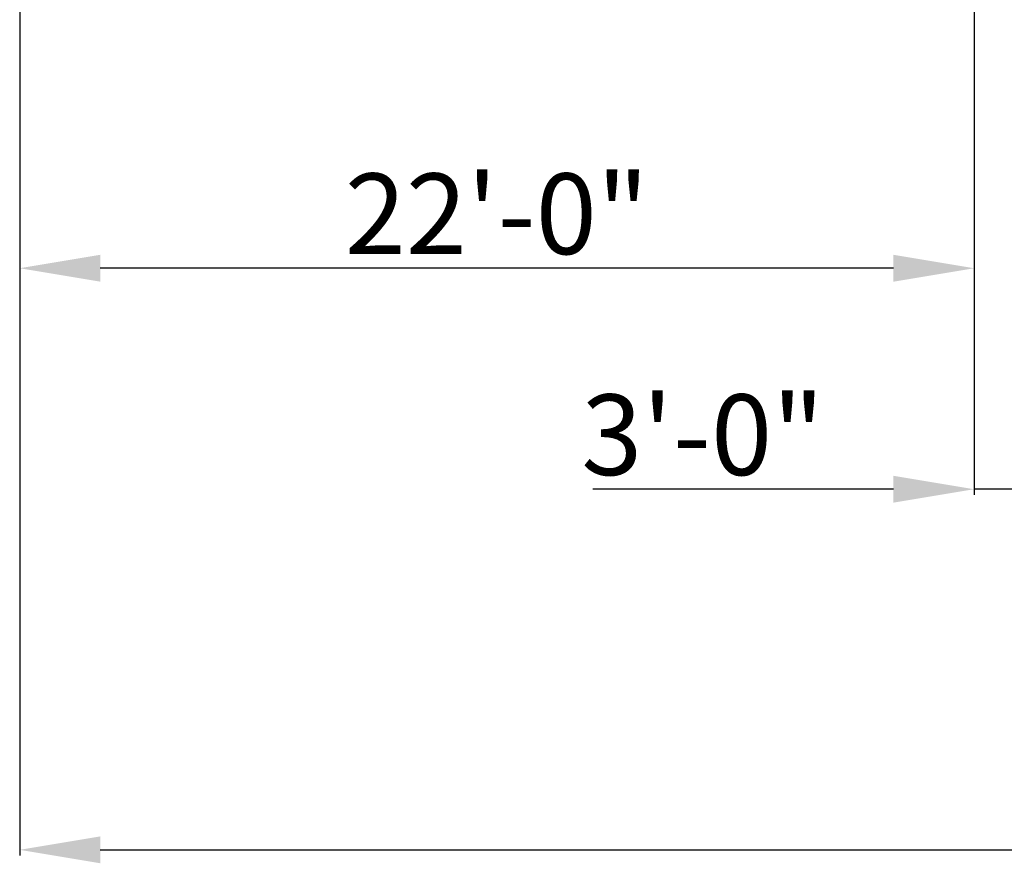
# Model space of a CAD drawing. Units: inches. Extents: x 2043 to 3177, y 1429 to 2563.
# Tile 1 of 14: x 2234 to 2453, y 1429 to 1617. Entities that reach past the tile are written whole.
import ezdxf

# ---------------------------------------------------------------- set-up
doc = ezdxf.new("R2010")
doc.units = ezdxf.units.IN
doc.layers.add('A-ANNO-DIMS', color=2, linetype='Continuous', lineweight=13)
doc.styles.get("Standard").update_dxf_attribs({"font": 'arial.ttf'})
doc.dimstyles.new('ISO-25', dxfattribs={"dimtxt": 18, "dimasz": 18, "dimexe": 1.25, "dimexo": 0.625, "dimtad": 1, "dimlunit": 3, "dimtxsty": 'Standard', "dimcen": 2.5, "dimadec": 0, "dimazin": 0, "dimtfac": 1, "dimtmove": 0, "dimatfit": 3, "dimfxl": 1, "dimarcsym": 0})

# ---------------------------------------------------------------- blocks, each defined once
blk = doc.blocks.new('*D23')
at = {"layer": 'A-ANNO-DIMS', "color": 0, "lineweight": -2, "transparency": 16777216}
for p, q in [((2446.74, 1641.77), (2446.74, 1511.06)), ((2482.49, 1641.77), (2482.49, 1511.06)), ((2428.74, 1512.31), (2361.66, 1512.31)), ((2482.49, 1512.31), (2446.74, 1512.31)), ((2500.49, 1512.31), (2518.49, 1512.31))]:
    blk.add_line(p, q, dxfattribs=at)
at = {"layer": 'A-ANNO-DIMS', "color": 0, "transparency": 16777216}
for points in [[(2428.74, 1515.31), (2428.74, 1509.31), (2446.74, 1512.31)], [(2500.49, 1515.31), (2500.49, 1509.31), (2482.49, 1512.31)]]:
    blk.add_solid(points, dxfattribs=at)
at = {"layer": 'Defpoints', "color": 0, "transparency": 16777216}
for p in [(2446.74, 1642.39), (2482.49, 1642.39), (2446.74, 1512.31)]:
    blk.add_point(p, dxfattribs=at)
at = {"layer": 'A-ANNO-DIMS', "color": 0, "transparency": 16777216, "insert": (2386.2, 1522.13), "char_height": 18, "attachment_point": 5}
blk.add_mtext('3\'-0"', dxfattribs=at)
blk = doc.blocks.new('*D24')
at = {"layer": 'A-ANNO-DIMS', "color": 0, "lineweight": -2, "transparency": 16777216}
for p, q in [((2233.74, 1633.77), (2233.74, 1560.37)), ((2446.74, 1633.77), (2446.74, 1560.37)), ((2428.74, 1561.62), (2251.74, 1561.62))]:
    blk.add_line(p, q, dxfattribs=at)
at = {"layer": 'A-ANNO-DIMS', "color": 0, "transparency": 16777216}
for points in [[(2251.74, 1564.62), (2251.74, 1558.62), (2233.74, 1561.62)], [(2428.74, 1564.62), (2428.74, 1558.62), (2446.74, 1561.62)]]:
    blk.add_solid(points, dxfattribs=at)
at = {"layer": 'Defpoints', "color": 0, "transparency": 16777216}
for p in [(2233.74, 1634.39), (2446.74, 1634.39), (2233.74, 1561.62)]:
    blk.add_point(p, dxfattribs=at)
at = {"layer": 'A-ANNO-DIMS', "color": 0, "transparency": 16777216, "insert": (2340.24, 1571.44), "char_height": 18, "attachment_point": 5}
blk.add_mtext('22\'-0"', dxfattribs=at)
blk = doc.blocks.new('*D29')
at = {"layer": 'A-ANNO-DIMS', "color": 0, "lineweight": -2, "transparency": 16777216}
for p, q in [((2233.74, 1633.77), (2233.74, 1430.58)), ((2980.74, 1633.77), (2980.74, 1430.58)), ((2251.74, 1431.83), (2962.74, 1431.83))]:
    blk.add_line(p, q, dxfattribs=at)
at = {"layer": 'A-ANNO-DIMS', "color": 0, "transparency": 16777216}
for points in [[(2251.74, 1434.83), (2251.74, 1428.83), (2233.74, 1431.83)], [(2962.74, 1434.83), (2962.74, 1428.83), (2980.74, 1431.83)]]:
    blk.add_solid(points, dxfattribs=at)
at = {"layer": 'Defpoints', "color": 0, "transparency": 16777216}
for p in [(2233.74, 1634.39), (2980.74, 1634.39), (2980.74, 1431.83)]:
    blk.add_point(p, dxfattribs=at)
at = {"layer": 'A-ANNO-DIMS', "color": 0, "transparency": 16777216, "insert": (2607.24, 1441.64), "char_height": 18, "attachment_point": 5}
blk.add_mtext('75\'-0"', dxfattribs=at)

msp = doc.modelspace()

# ---------------------------------------------------------------- dimensions: what is measured, and where the dimension line sits
at = {"layer": 'A-ANNO-DIMS'}
for base, p1, p2, text, picture, middle in [((2446.745, 1512.311), (2482.495, 1642.393), (2446.745, 1642.393), '3\'-0"', '*D23', (2386.201, 1522.132)), ((2233.745, 1561.62), (2446.745, 1634.393), (2233.745, 1634.393), '22\'-0"', '*D24', (2340.245, 1571.436)), ((2980.745, 1431.826), (2233.745, 1634.393), (2980.745, 1634.393), '75\'-0"', '*D29', (2607.245, 1441.642))]:
    dim = msp.add_linear_dim(base=base, p1=p1, p2=p2, text=text, dimstyle='ISO-25', override={"dimclrd": 0, "dimclre": 0, "dimclrt": 0}, dxfattribs=at)
    dim.commit()
    dim.dimension.update_dxf_attribs({"geometry": picture, "text_midpoint": middle})

doc.saveas('drawing.dxf')
